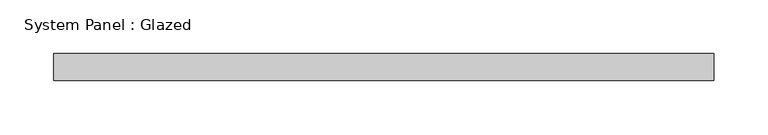
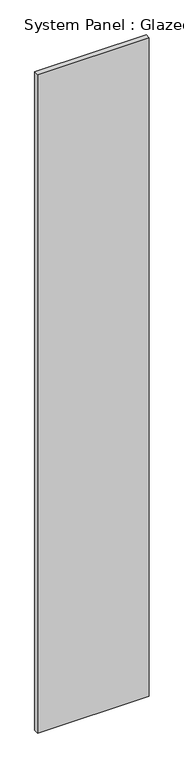
"""IFC4 building model written with IfcOpenShell, lengths in millimetres: plate geometry, System Panel : Glazed."""

from ifc_helpers import new_model, si_unit, origin, origin_with_axes, place, context, project, spatial, polyline, outline, extrude, source, transform, mapped, element, save


def system_panel_glazed_d7bd2e6f(model_context):
    return source(origin(), model_context, "Body", "SweptSolid", [
        extrude(outline(polyline([(307.6922868, 19.05), (-307.6922868, 19.05), (-307.6922868, 44.45), (307.6922868, 44.45), (307.6922868, 19.05)])), origin_with_axes(), (0.0, 0.0, 1.0), 3835.4),
    ])


if __name__ == "__main__":
    model = new_model("IFC4")
    model_context = context("Model", 3, world=origin())
    ifc_project = project(units=[si_unit("LENGTHUNIT", "METRE", prefix="MILLI")], contexts=[model_context])
    site = spatial("IfcSite", under=ifc_project)
    building = spatial("IfcBuilding", under=site)
    placement = place(None, origin())
    system_panel_glazed_shape = system_panel_glazed_d7bd2e6f(model_context)
    element("IfcPlate", 1, ObjectType="System Panel : Glazed", at=placement, inside=building, context=model_context, shape_type="MappedRepresentation", body=[
        mapped(system_panel_glazed_shape, transform((0.0, 0.0, 0.0), x_axis=(1.0, 0.0, 0.0), y_axis=(0.0, 1.0, 0.0), z_axis=(0.0, 0.0, 1.0))),
    ])
    save(model, "model.ifc")

# Revit data of these elements
# Type "System Panel : Glazed"
#   Construction Type Id = "GSP4R"
#   Analytic Construction = "1/8 in Pilkington single glazing"
#   Visual Light Transmittance = 0.9
#   Solar Heat Gain Coefficient = 0.86
#   Heat Transfer Coefficient (U) = 1.18115 BTU/(h·ft²·°F)
# Element 1 (IfcPlate, "System Panel : Glazed")
#   Materials on its faces: "Glass"
# Materials
#   "Glass": class "Glass", colour RGB 0 128 192, transparency 0.75, Description = "Soda Lime Glass", Cost = 0
